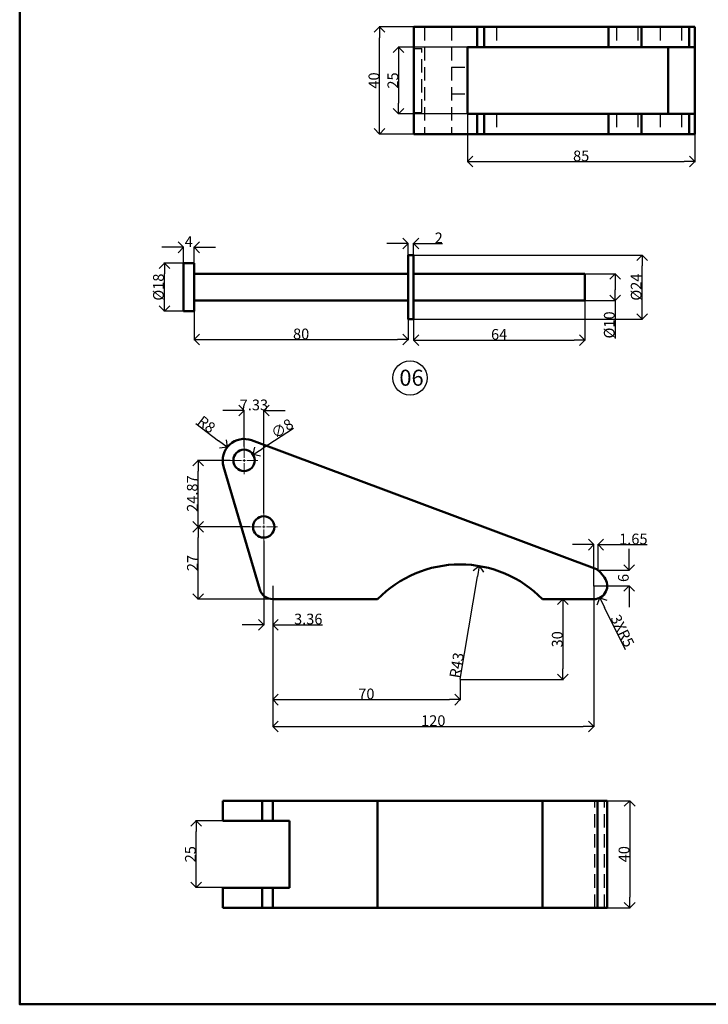
# Model space of a CAD drawing. Units: millimetres. Extents: x 45 to 546, y 51 to 638.
# Tile 1 of 4: x 45 to 303, y 51 to 419. Entities that reach past the tile are written whole.
import ezdxf

# ---------------------------------------------------------------- set-up
doc = ezdxf.new("R2010")
doc.units = ezdxf.units.MM
doc.header["$MEASUREMENT"] = 0
doc.linetypes.add('CENTER2', pattern=[1.125, 0.75, -0.125, 0.125, -0.125])
doc.linetypes.add('HIDDEN', pattern=[0.375, 0.25, -0.125])
for name, color, linetype, lineweight in [('M-CNTR', 1, 'CENTER2', 18), ('M-DIMS', 2, 'Continuous', 25), ('M-HIDN', 8, 'HIDDEN', 25), ('M-OUTL', 7, 'Continuous', 50), ('M-TEXT', 7, 'Continuous', 25), ('M-TTLB', 7, 'Continuous', 50)]:
    doc.layers.add(name, color=color, linetype=linetype, lineweight=lineweight)
doc.styles.get("Standard").update_dxf_attribs({"font": 'arial.ttf'})
doc.dimstyles.get("Standard").update_dxf_attribs({"dimtxt": 4, "dimasz": 4, "dimexe": 0.18, "dimexo": 0.0625, "dimgap": 0.09, "dimtad": 1, "dimdec": 0, "dimzin": 0, "dimdsep": 46, "dimtxsty": 'Standard', "dimblk": 'OPEN90', "dimcen": 0.09, "dimclre": 251, "dimadec": 0, "dimazin": 0, "dimtfac": 1, "dimtdec": 0, "dimtofl": 0, "dimtmove": 0, "dimatfit": 3, "dimfxl": 1, "dimtolj": 1, "dimtzin": 0, "dimarcsym": 0})

# ---------------------------------------------------------------- blocks, each defined once
blk = doc.blocks.new('_Open90')
at = {"color": 0, "linetype": 'ByBlock', "lineweight": -2}
for p, q in [((0, 0), (-1, 0)), ((-0.5, 0.5), (0, 0)), ((0, 0), (-0.5, -0.5))]:
    blk.add_line(p, q, dxfattribs=at)
blk = doc.blocks.new('*D28')
at = {"layer": 'Defpoints', "color": 0, "transparency": 16777216}
for p in [(179.84, 416.24), (192.68, 416.24), (192.68, 376.24)]:
    blk.add_point(p, dxfattribs=at)
at = {"layer": 'M-DIMS', "color": 0, "lineweight": -2, "transparency": 16777216}
for p, q in [((192.61, 416.24), (179.66, 416.24)), ((179.84, 380.24), (179.84, 412.24)), ((192.61, 376.24), (179.66, 376.24))]:
    blk.add_line(p, q, dxfattribs=at)
at = {"layer": 'M-DIMS', "color": 0, "lineweight": -2, "transparency": 16777216, "xscale": 4, "yscale": 4, "zscale": 4}
for p, rotation in [((179.84, 416.24), 90), ((179.84, 376.24), 270)]:
    blk.add_blockref('_Open90', p, dxfattribs=dict(at, rotation=rotation))
at = {"layer": 'M-DIMS', "color": 0, "transparency": 16777216, "insert": (177.71, 396.24), "char_height": 4, "attachment_point": 5, "rotation": 90}
blk.add_mtext('\\A1;40', dxfattribs=at)
blk = doc.blocks.new('*D29')
at = {"layer": 'Defpoints', "color": 0, "transparency": 16777216}
for p in [(212.68, 408.74), (186.92, 383.74), (212.68, 383.74)]:
    blk.add_point(p, dxfattribs=at)
at = {"layer": 'M-DIMS', "color": 0, "lineweight": -2, "transparency": 16777216}
for p, q in [((212.61, 408.74), (186.74, 408.74)), ((186.92, 404.74), (186.92, 387.74)), ((212.61, 383.74), (186.74, 383.74))]:
    blk.add_line(p, q, dxfattribs=at)
at = {"layer": 'M-DIMS', "color": 0, "lineweight": -2, "transparency": 16777216, "xscale": 4, "yscale": 4, "zscale": 4}
for p, rotation in [((186.92, 408.74), 90), ((186.92, 383.74), 270)]:
    blk.add_blockref('_Open90', p, dxfattribs=dict(at, rotation=rotation))
at = {"layer": 'M-DIMS', "color": 0, "transparency": 16777216, "insert": (184.79, 396.24), "char_height": 4, "attachment_point": 5, "rotation": 90}
blk.add_mtext('\\A1;25', dxfattribs=at)
blk = doc.blocks.new('*D30')
at = {"layer": 'Defpoints', "color": 0, "transparency": 16777216}
for p in [(212.68, 383.74), (297.68, 383.74), (297.68, 365.93)]:
    blk.add_point(p, dxfattribs=at)
at = {"layer": 'M-DIMS', "color": 0, "lineweight": -2, "transparency": 16777216}
for p, q in [((212.68, 383.68), (212.68, 365.75)), ((297.68, 383.68), (297.68, 365.75)), ((216.68, 365.93), (293.68, 365.93))]:
    blk.add_line(p, q, dxfattribs=at)
at = {"layer": 'M-DIMS', "color": 0, "lineweight": -2, "transparency": 16777216, "xscale": 4, "yscale": 4, "zscale": 4, "rotation": 180}
blk.add_blockref('_Open90', (212.68, 365.93), dxfattribs=at)
at = {"layer": 'M-DIMS', "color": 0, "lineweight": -2, "transparency": 16777216, "xscale": 4, "yscale": 4, "zscale": 4}
blk.add_blockref('_Open90', (297.68, 365.93), dxfattribs=at)
at = {"layer": 'M-DIMS', "color": 0, "transparency": 16777216, "insert": (255.18, 368.06), "char_height": 4, "attachment_point": 5}
blk.add_mtext('\\A1;85', dxfattribs=at)
blk = doc.blocks.new('*D77')
at = {"layer": 'Defpoints', "color": 0, "transparency": 16777216}
for p in [(99.44, 328.03), (106.53, 328.03), (106.53, 310.03)]:
    blk.add_point(p, dxfattribs=at)
at = {"layer": 'M-DIMS', "color": 0, "lineweight": -2, "transparency": 16777216}
for p, q in [((106.46, 328.03), (99.26, 328.03)), ((99.44, 314.03), (99.44, 324.03)), ((106.46, 310.03), (99.26, 310.03))]:
    blk.add_line(p, q, dxfattribs=at)
at = {"layer": 'M-DIMS', "color": 0, "lineweight": -2, "transparency": 16777216, "xscale": 4, "yscale": 4, "zscale": 4}
for p, rotation in [((99.44, 328.03), 90), ((99.44, 310.03), 270)]:
    blk.add_blockref('_Open90', p, dxfattribs=dict(at, rotation=rotation))
at = {"layer": 'M-DIMS', "color": 0, "transparency": 16777216, "insert": (97.2, 319.03), "char_height": 4, "attachment_point": 5, "rotation": 90}
blk.add_mtext('\\A1;%%C18', dxfattribs=at)
blk = doc.blocks.new('*D78')
at = {"layer": 'Defpoints', "color": 0, "transparency": 16777216}
for p in [(110.53, 333.9), (106.53, 328.03), (110.53, 328.03)]:
    blk.add_point(p, dxfattribs=at)
at = {"layer": 'M-DIMS', "color": 0, "lineweight": -2, "transparency": 16777216}
for p, q in [((102.53, 333.9), (98.53, 333.9)), ((106.53, 328.09), (106.53, 334.08)), ((110.53, 328.09), (110.53, 334.08)), ((114.53, 333.9), (118.53, 333.9))]:
    blk.add_line(p, q, dxfattribs=at)
at = {"layer": 'M-DIMS', "color": 0, "lineweight": -2, "transparency": 16777216, "xscale": 4, "yscale": 4, "zscale": 4}
blk.add_blockref('_Open90', (106.53, 333.9), dxfattribs=at)
at = {"layer": 'M-DIMS', "color": 0, "lineweight": -2, "transparency": 16777216, "xscale": 4, "yscale": 4, "zscale": 4, "rotation": 180}
blk.add_blockref('_Open90', (110.53, 333.9), dxfattribs=at)
at = {"layer": 'M-DIMS', "color": 0, "transparency": 16777216, "insert": (108.53, 335.99), "char_height": 4, "attachment_point": 5}
blk.add_mtext('\\A1;4', dxfattribs=at)
blk = doc.blocks.new('*D79')
at = {"layer": 'Defpoints', "color": 0, "transparency": 16777216}
for p in [(192.53, 335.33), (190.53, 331.03), (192.53, 331.03)]:
    blk.add_point(p, dxfattribs=at)
at = {"layer": 'M-DIMS', "color": 0, "lineweight": -2, "transparency": 16777216}
for p, q in [((186.53, 335.33), (182.53, 335.33)), ((190.53, 331.09), (190.53, 335.51)), ((192.53, 331.09), (192.53, 335.51)), ((196.53, 335.33), (203.36, 335.33))]:
    blk.add_line(p, q, dxfattribs=at)
at = {"layer": 'M-DIMS', "color": 0, "lineweight": -2, "transparency": 16777216, "xscale": 4, "yscale": 4, "zscale": 4}
blk.add_blockref('_Open90', (190.53, 335.33), dxfattribs=at)
at = {"layer": 'M-DIMS', "color": 0, "lineweight": -2, "transparency": 16777216, "xscale": 4, "yscale": 4, "zscale": 4, "rotation": 180}
blk.add_blockref('_Open90', (192.53, 335.33), dxfattribs=at)
at = {"layer": 'M-DIMS', "color": 0, "transparency": 16777216, "insert": (201.94, 337.43), "char_height": 4, "attachment_point": 5}
blk.add_mtext('\\A1;2', dxfattribs=at)
blk = doc.blocks.new('*D80')
at = {"layer": 'Defpoints', "color": 0, "transparency": 16777216}
for p in [(110.53, 310.03), (190.53, 307.03), (190.53, 299.42)]:
    blk.add_point(p, dxfattribs=at)
at = {"layer": 'M-DIMS', "color": 0, "lineweight": -2, "transparency": 16777216}
for p, q in [((110.53, 309.96), (110.53, 299.24)), ((190.53, 306.96), (190.53, 299.24)), ((114.53, 299.42), (186.53, 299.42))]:
    blk.add_line(p, q, dxfattribs=at)
at = {"layer": 'M-DIMS', "color": 0, "lineweight": -2, "transparency": 16777216, "xscale": 4, "yscale": 4, "zscale": 4, "rotation": 180}
blk.add_blockref('_Open90', (110.53, 299.42), dxfattribs=at)
at = {"layer": 'M-DIMS', "color": 0, "lineweight": -2, "transparency": 16777216, "xscale": 4, "yscale": 4, "zscale": 4}
blk.add_blockref('_Open90', (190.53, 299.42), dxfattribs=at)
at = {"layer": 'M-DIMS', "color": 0, "transparency": 16777216, "insert": (150.53, 301.55), "char_height": 4, "attachment_point": 5}
blk.add_mtext('\\A1;80', dxfattribs=at)
blk = doc.blocks.new('*D81')
at = {"layer": 'Defpoints', "color": 0, "transparency": 16777216}
for p in [(256.53, 314.03), (192.53, 307.03), (256.53, 299.24)]:
    blk.add_point(p, dxfattribs=at)
at = {"layer": 'M-DIMS', "color": 0, "lineweight": -2, "transparency": 16777216}
for p, q in [((256.53, 313.96), (256.53, 299.06)), ((192.53, 306.96), (192.53, 299.06)), ((196.53, 299.24), (252.53, 299.24))]:
    blk.add_line(p, q, dxfattribs=at)
at = {"layer": 'M-DIMS', "color": 0, "lineweight": -2, "transparency": 16777216, "xscale": 4, "yscale": 4, "zscale": 4, "rotation": 180}
blk.add_blockref('_Open90', (192.53, 299.24), dxfattribs=at)
at = {"layer": 'M-DIMS', "color": 0, "lineweight": -2, "transparency": 16777216, "xscale": 4, "yscale": 4, "zscale": 4}
blk.add_blockref('_Open90', (256.53, 299.24), dxfattribs=at)
at = {"layer": 'M-DIMS', "color": 0, "transparency": 16777216, "insert": (224.53, 301.37), "char_height": 4, "attachment_point": 5}
blk.add_mtext('\\A1;64', dxfattribs=at)
blk = doc.blocks.new('*D82')
at = {"layer": 'Defpoints', "color": 0, "transparency": 16777216}
for p in [(256.53, 324.03), (256.53, 314.03), (267.91, 314.03)]:
    blk.add_point(p, dxfattribs=at)
at = {"layer": 'M-DIMS', "color": 0, "lineweight": -2, "transparency": 16777216}
for p, q in [((256.59, 324.03), (268.09, 324.03)), ((267.91, 320.03), (267.91, 318.03)), ((256.59, 314.03), (268.09, 314.03)), ((267.91, 314.03), (267.91, 299.78))]:
    blk.add_line(p, q, dxfattribs=at)
at = {"layer": 'M-DIMS', "color": 0, "lineweight": -2, "transparency": 16777216, "xscale": 4, "yscale": 4, "zscale": 4}
for p, rotation in [((267.91, 324.03), 90), ((267.91, 314.03), 270)]:
    blk.add_blockref('_Open90', p, dxfattribs=dict(at, rotation=rotation))
at = {"layer": 'M-DIMS', "color": 0, "transparency": 16777216, "insert": (265.67, 304.9), "char_height": 4, "attachment_point": 5, "rotation": 90}
blk.add_mtext('\\A1;%%C10', dxfattribs=at)
blk = doc.blocks.new('*D83')
at = {"layer": 'Defpoints', "color": 0, "transparency": 16777216}
for p in [(192.53, 331.03), (277.97, 331.03), (192.53, 307.03)]:
    blk.add_point(p, dxfattribs=at)
at = {"layer": 'M-DIMS', "color": 0, "lineweight": -2, "transparency": 16777216}
for p, q in [((192.59, 331.03), (278.15, 331.03)), ((277.97, 311.03), (277.97, 327.03)), ((192.59, 307.03), (278.15, 307.03))]:
    blk.add_line(p, q, dxfattribs=at)
at = {"layer": 'M-DIMS', "color": 0, "lineweight": -2, "transparency": 16777216, "xscale": 4, "yscale": 4, "zscale": 4}
for p, rotation in [((277.97, 331.03), 90), ((277.97, 307.03), 270)]:
    blk.add_blockref('_Open90', p, dxfattribs=dict(at, rotation=rotation))
at = {"layer": 'M-DIMS', "color": 0, "transparency": 16777216, "insert": (275.73, 319.03), "char_height": 4, "attachment_point": 5, "rotation": 90}
blk.add_mtext('\\A1;%%C24', dxfattribs=at)
blk = doc.blocks.new('*U84')
at = {"layer": 'M-CNTR', "color": 0, "transparency": 16777216}
for p, q in [((0, 1), (0, 5.12)), ((-5.12, 0), (-1, 0)), ((1, 0), (5.12, 0)), ((0, -5.12), (0, -1))]:
    blk.add_line(p, q, dxfattribs=at)
at = {"layer": 'M-CNTR', "color": 0, "linetype": 'Continuous', "transparency": 16777216}
for p, q in [((-0.5, 0), (0.5, 0)), ((0, -0.5), (0, 0.5))]:
    blk.add_line(p, q, dxfattribs=at)
blk = doc.blocks.new('*U85')
at = {"layer": 'M-CNTR', "color": 0, "transparency": 16777216}
for p, q in [((0, 1), (0, 5.12)), ((-5.12, 0), (-1, 0)), ((1, 0), (5.12, 0)), ((0, -5.12), (0, -1))]:
    blk.add_line(p, q, dxfattribs=at)
at = {"layer": 'M-CNTR', "color": 0, "linetype": 'Continuous', "transparency": 16777216}
for p, q in [((-0.5, 0), (0.5, 0)), ((0, -0.5), (0, 0.5))]:
    blk.add_line(p, q, dxfattribs=at)
blk = doc.blocks.new('*D86')
at = {"layer": 'Defpoints', "color": 0, "transparency": 16777216}
for p in [(112, 229.43), (131.43, 229.43), (139.91, 202.43)]:
    blk.add_point(p, dxfattribs=at)
at = {"layer": 'M-DIMS', "color": 0, "lineweight": -2, "transparency": 16777216}
for p, q in [((131.37, 229.43), (111.82, 229.43)), ((112, 206.43), (112, 225.43)), ((139.85, 202.43), (111.82, 202.43))]:
    blk.add_line(p, q, dxfattribs=at)
at = {"layer": 'M-DIMS', "color": 0, "lineweight": -2, "transparency": 16777216, "xscale": 4, "yscale": 4, "zscale": 4}
for p, rotation in [((112, 229.43), 90), ((112, 202.43), 270)]:
    blk.add_blockref('_Open90', p, dxfattribs=dict(at, rotation=rotation))
at = {"layer": 'M-DIMS', "color": 0, "transparency": 16777216, "insert": (109.9, 215.93), "char_height": 4, "attachment_point": 5, "rotation": 90}
blk.add_mtext('\\A1;27', dxfattribs=at)
blk = doc.blocks.new('*D87')
at = {"layer": 'Defpoints', "color": 0, "transparency": 16777216}
for p in [(112, 254.3), (124.1, 254.3), (131.43, 229.43)]:
    blk.add_point(p, dxfattribs=at)
at = {"layer": 'M-DIMS', "color": 0, "lineweight": -2, "transparency": 16777216}
for p, q in [((124.04, 254.3), (111.82, 254.3)), ((112, 233.43), (112, 250.3)), ((131.37, 229.43), (111.82, 229.43))]:
    blk.add_line(p, q, dxfattribs=at)
at = {"layer": 'M-DIMS', "color": 0, "lineweight": -2, "transparency": 16777216, "xscale": 4, "yscale": 4, "zscale": 4}
for p, rotation in [((112, 254.3), 90), ((112, 229.43), 270)]:
    blk.add_blockref('_Open90', p, dxfattribs=dict(at, rotation=rotation))
at = {"layer": 'M-DIMS', "color": 0, "transparency": 16777216, "insert": (109.86, 241.87), "char_height": 4, "attachment_point": 5, "rotation": 90}
blk.add_mtext('\\A1;24.87', dxfattribs=at)
blk = doc.blocks.new('*D88')
at = {"layer": 'Defpoints', "color": 0, "transparency": 16777216}
for p in [(129.22, 272.89), (129.22, 259.42), (136.55, 234.55)]:
    blk.add_point(p, dxfattribs=at)
at = {"layer": 'M-DIMS', "color": 0, "lineweight": -2, "transparency": 16777216}
for p, q in [((125.22, 272.89), (121.22, 272.89)), ((129.22, 259.49), (129.22, 273.07)), ((136.55, 234.62), (136.55, 273.07)), ((140.55, 272.89), (144.55, 272.89))]:
    blk.add_line(p, q, dxfattribs=at)
at = {"layer": 'M-DIMS', "color": 0, "lineweight": -2, "transparency": 16777216, "xscale": 4, "yscale": 4, "zscale": 4}
blk.add_blockref('_Open90', (129.22, 272.89), dxfattribs=at)
at = {"layer": 'M-DIMS', "color": 0, "lineweight": -2, "transparency": 16777216, "xscale": 4, "yscale": 4, "zscale": 4, "rotation": 180}
blk.add_blockref('_Open90', (136.55, 272.89), dxfattribs=at)
at = {"layer": 'M-DIMS', "color": 0, "transparency": 16777216, "insert": (132.88, 275.02), "char_height": 4, "attachment_point": 5}
blk.add_mtext('\\A1;7.33', dxfattribs=at)
blk = doc.blocks.new('*D89')
at = {"layer": 'Defpoints', "color": 0, "transparency": 16777216}
for p in [(122.86, 259.17), (129.22, 254.3)]:
    blk.add_point(p, dxfattribs=at)
at = {"layer": 'M-DIMS', "color": 0, "lineweight": -2, "transparency": 16777216}
for p, q in [((111.24, 268.06), (119.69, 261.6)), ((129.13, 254.3), (129.31, 254.3)), ((129.22, 254.21), (129.22, 254.39))]:
    blk.add_line(p, q, dxfattribs=at)
at = {"layer": 'M-DIMS', "color": 0, "lineweight": -2, "transparency": 16777216, "xscale": 4, "yscale": 4, "zscale": 4, "rotation": 322.5817597606711}
blk.add_blockref('_Open90', (122.86, 259.17), dxfattribs=at)
at = {"layer": 'M-DIMS', "color": 0, "transparency": 16777216, "insert": (115.17, 267.74), "char_height": 4, "attachment_point": 5, "rotation": 322.5818}
blk.add_mtext('\\A1;R8', dxfattribs=at)
blk = doc.blocks.new('*D90')
at = {"layer": 'Defpoints', "color": 0, "transparency": 16777216}
for p in [(132.58, 256.48), (125.86, 252.13)]:
    blk.add_point(p, dxfattribs=at)
at = {"layer": 'M-DIMS', "color": 0, "lineweight": -2, "transparency": 16777216}
for p, q in [((147.67, 266.24), (135.93, 258.65)), ((129.13, 254.3), (129.31, 254.3)), ((129.22, 254.21), (129.22, 254.39))]:
    blk.add_line(p, q, dxfattribs=at)
at = {"layer": 'M-DIMS', "color": 0, "lineweight": -2, "transparency": 16777216, "xscale": 4, "yscale": 4, "zscale": 4, "rotation": 212.9103670149516}
blk.add_blockref('_Open90', (132.58, 256.48), dxfattribs=at)
at = {"layer": 'M-DIMS', "color": 0, "transparency": 16777216, "insert": (143.44, 266.18), "char_height": 4, "attachment_point": 5, "rotation": 32.9104}
blk.add_mtext('\\A1;∅8', dxfattribs=at)
blk = doc.blocks.new('*D91')
at = {"layer": 'Defpoints', "color": 0, "transparency": 16777216}
for p in [(136.55, 224.31), (139.91, 207.43), (139.91, 192.87)]:
    blk.add_point(p, dxfattribs=at)
at = {"layer": 'M-DIMS', "color": 0, "lineweight": -2, "transparency": 16777216}
for p, q in [((136.55, 224.25), (136.55, 192.69)), ((139.91, 207.37), (139.91, 192.69)), ((132.55, 192.87), (128.55, 192.87)), ((143.91, 192.87), (158.47, 192.87))]:
    blk.add_line(p, q, dxfattribs=at)
at = {"layer": 'M-DIMS', "color": 0, "lineweight": -2, "transparency": 16777216, "xscale": 4, "yscale": 4, "zscale": 4}
blk.add_blockref('_Open90', (136.55, 192.87), dxfattribs=at)
at = {"layer": 'M-DIMS', "color": 0, "lineweight": -2, "transparency": 16777216, "xscale": 4, "yscale": 4, "zscale": 4, "rotation": 180}
blk.add_blockref('_Open90', (139.91, 192.87), dxfattribs=at)
at = {"layer": 'M-DIMS', "color": 0, "transparency": 16777216, "insert": (153.19, 195.01), "char_height": 4, "attachment_point": 5}
blk.add_mtext('\\A1;3.36', dxfattribs=at)
blk = doc.blocks.new('*D92')
at = {"layer": 'Defpoints', "color": 0, "transparency": 16777216}
for p in [(139.91, 207.43), (209.91, 172.43), (209.91, 164.89)]:
    blk.add_point(p, dxfattribs=at)
at = {"layer": 'M-DIMS', "color": 0, "lineweight": -2, "transparency": 16777216}
for p, q in [((139.91, 207.37), (139.91, 164.71)), ((209.91, 172.37), (209.91, 164.71)), ((143.91, 164.89), (205.91, 164.89))]:
    blk.add_line(p, q, dxfattribs=at)
at = {"layer": 'M-DIMS', "color": 0, "lineweight": -2, "transparency": 16777216, "xscale": 4, "yscale": 4, "zscale": 4, "rotation": 180}
blk.add_blockref('_Open90', (139.91, 164.89), dxfattribs=at)
at = {"layer": 'M-DIMS', "color": 0, "lineweight": -2, "transparency": 16777216, "xscale": 4, "yscale": 4, "zscale": 4}
blk.add_blockref('_Open90', (209.91, 164.89), dxfattribs=at)
at = {"layer": 'M-DIMS', "color": 0, "transparency": 16777216, "insert": (174.91, 167.03), "char_height": 4, "attachment_point": 5}
blk.add_mtext('\\A1;70', dxfattribs=at)
blk = doc.blocks.new('*D93')
at = {"layer": 'Defpoints', "color": 0, "transparency": 16777216}
for p in [(245.97, 202.43), (209.91, 172.43), (248.37, 172.43)]:
    blk.add_point(p, dxfattribs=at)
at = {"layer": 'M-DIMS', "color": 0, "lineweight": -2, "transparency": 16777216}
for p, q in [((246.04, 202.43), (248.55, 202.43)), ((248.37, 198.43), (248.37, 176.43)), ((209.97, 172.43), (248.55, 172.43))]:
    blk.add_line(p, q, dxfattribs=at)
at = {"layer": 'M-DIMS', "color": 0, "lineweight": -2, "transparency": 16777216, "xscale": 4, "yscale": 4, "zscale": 4}
for p, rotation in [((248.37, 202.43), 90), ((248.37, 172.43), 270)]:
    blk.add_blockref('_Open90', p, dxfattribs=dict(at, rotation=rotation))
at = {"layer": 'M-DIMS', "color": 0, "transparency": 16777216, "insert": (246.23, 187.43), "char_height": 4, "attachment_point": 5, "rotation": 90}
blk.add_mtext('\\A1;30', dxfattribs=at)
blk = doc.blocks.new('*D94')
at = {"layer": 'Defpoints', "color": 0, "transparency": 16777216}
for p in [(139.91, 207.43), (259.91, 207.43), (259.91, 154.91)]:
    blk.add_point(p, dxfattribs=at)
at = {"layer": 'M-DIMS', "color": 0, "lineweight": -2, "transparency": 16777216}
for p, q in [((139.91, 207.37), (139.91, 154.73)), ((259.91, 207.37), (259.91, 154.73)), ((143.91, 154.91), (255.91, 154.91))]:
    blk.add_line(p, q, dxfattribs=at)
at = {"layer": 'M-DIMS', "color": 0, "lineweight": -2, "transparency": 16777216, "xscale": 4, "yscale": 4, "zscale": 4, "rotation": 180}
blk.add_blockref('_Open90', (139.91, 154.91), dxfattribs=at)
at = {"layer": 'M-DIMS', "color": 0, "lineweight": -2, "transparency": 16777216, "xscale": 4, "yscale": 4, "zscale": 4}
blk.add_blockref('_Open90', (259.91, 154.91), dxfattribs=at)
at = {"layer": 'M-DIMS', "color": 0, "transparency": 16777216, "insert": (199.91, 157.04), "char_height": 4, "attachment_point": 5}
blk.add_mtext('\\A1;120', dxfattribs=at)
blk = doc.blocks.new('*D95')
at = {"layer": 'Defpoints', "color": 0, "transparency": 16777216}
for p in [(217.1, 214.83), (209.91, 172.43)]:
    blk.add_point(p, dxfattribs=at)
at = {"layer": 'M-DIMS', "color": 0, "lineweight": -2, "transparency": 16777216}
blk.add_line((209.93, 172.57), (216.43, 210.89), dxfattribs=at)
at = {"layer": 'M-DIMS', "color": 0, "lineweight": -2, "transparency": 16777216, "xscale": 4, "yscale": 4, "zscale": 4, "rotation": 80.37551850452407}
blk.add_blockref('_Open90', (217.1, 214.83), dxfattribs=at)
at = {"layer": 'M-DIMS', "color": 0, "transparency": 16777216, "insert": (208.64, 177.73), "char_height": 4, "attachment_point": 5, "rotation": 80.3755}
blk.add_mtext('\\A1;R43', dxfattribs=at)
blk = doc.blocks.new('*D96')
at = {"layer": 'Defpoints', "color": 0, "transparency": 16777216}
for p in [(261.45, 213.29), (273.08, 213.29), (259.91, 207.43)]:
    blk.add_point(p, dxfattribs=at)
at = {"layer": 'M-DIMS', "color": 0, "lineweight": -2, "transparency": 16777216}
for p, q in [((273.08, 217.29), (273.08, 221.29)), ((261.51, 213.29), (273.26, 213.29)), ((259.97, 207.43), (273.26, 207.43)), ((273.08, 203.43), (273.08, 199.43))]:
    blk.add_line(p, q, dxfattribs=at)
at = {"layer": 'M-DIMS', "color": 0, "lineweight": -2, "transparency": 16777216, "xscale": 4, "yscale": 4, "zscale": 4}
for p, rotation in [((273.08, 213.29), 270), ((273.08, 207.43), 90)]:
    blk.add_blockref('_Open90', p, dxfattribs=dict(at, rotation=rotation))
at = {"layer": 'M-DIMS', "color": 0, "transparency": 16777216, "insert": (270.95, 210.36), "char_height": 4, "attachment_point": 5, "rotation": 90}
blk.add_mtext('\\A1;6', dxfattribs=at)
blk = doc.blocks.new('*D97')
at = {"layer": 'Defpoints', "color": 0, "transparency": 16777216}
for p in [(261.56, 222.8), (261.56, 213.2), (259.91, 207.43)]:
    blk.add_point(p, dxfattribs=at)
at = {"layer": 'M-DIMS', "color": 0, "lineweight": -2, "transparency": 16777216}
for p, q in [((255.91, 222.8), (251.91, 222.8)), ((259.91, 207.5), (259.91, 222.98)), ((261.56, 213.27), (261.56, 222.98)), ((265.56, 222.8), (279.78, 222.8))]:
    blk.add_line(p, q, dxfattribs=at)
at = {"layer": 'M-DIMS', "color": 0, "lineweight": -2, "transparency": 16777216, "xscale": 4, "yscale": 4, "zscale": 4}
blk.add_blockref('_Open90', (259.91, 222.8), dxfattribs=at)
at = {"layer": 'M-DIMS', "color": 0, "lineweight": -2, "transparency": 16777216, "xscale": 4, "yscale": 4, "zscale": 4, "rotation": 180}
blk.add_blockref('_Open90', (261.56, 222.8), dxfattribs=at)
at = {"layer": 'M-DIMS', "color": 0, "transparency": 16777216, "insert": (274.67, 224.93), "char_height": 4, "attachment_point": 5}
blk.add_mtext('\\A1;1.65', dxfattribs=at)
blk = doc.blocks.new('*D98')
at = {"layer": 'Defpoints', "color": 0, "transparency": 16777216}
for p in [(259.91, 207.43), (262.12, 202.95)]:
    blk.add_point(p, dxfattribs=at)
at = {"layer": 'M-DIMS', "color": 0, "lineweight": -2, "transparency": 16777216}
for p, q in [((259.82, 207.43), (260, 207.43)), ((259.91, 207.34), (259.91, 207.52)), ((271.74, 183.5), (263.9, 199.37))]:
    blk.add_line(p, q, dxfattribs=at)
at = {"layer": 'M-DIMS', "color": 0, "lineweight": -2, "transparency": 16777216, "xscale": 4, "yscale": 4, "zscale": 4, "rotation": 116.3040513047438}
blk.add_blockref('_Open90', (262.12, 202.95), dxfattribs=at)
at = {"layer": 'M-DIMS', "color": 0, "transparency": 16777216, "insert": (270.62, 190.59), "char_height": 4, "attachment_point": 5, "rotation": 296.3041}
blk.add_mtext('\\A1;3XR5', dxfattribs=at)
blk = doc.blocks.new('*D99')
at = {"layer": 'Defpoints', "color": 0, "transparency": 16777216}
for p in [(111.27, 119.64), (121.22, 119.64), (121.22, 94.64)]:
    blk.add_point(p, dxfattribs=at)
at = {"layer": 'M-DIMS', "color": 0, "lineweight": -2, "transparency": 16777216}
for p, q in [((121.16, 119.64), (111.09, 119.64)), ((111.27, 98.64), (111.27, 115.64)), ((121.16, 94.64), (111.09, 94.64))]:
    blk.add_line(p, q, dxfattribs=at)
at = {"layer": 'M-DIMS', "color": 0, "lineweight": -2, "transparency": 16777216, "xscale": 4, "yscale": 4, "zscale": 4}
for p, rotation in [((111.27, 119.64), 90), ((111.27, 94.64), 270)]:
    blk.add_blockref('_Open90', p, dxfattribs=dict(at, rotation=rotation))
at = {"layer": 'M-DIMS', "color": 0, "transparency": 16777216, "insert": (109.13, 107.14), "char_height": 4, "attachment_point": 5, "rotation": 90}
blk.add_mtext('\\A1;25', dxfattribs=at)
blk = doc.blocks.new('*D100')
at = {"layer": 'Defpoints', "color": 0, "transparency": 16777216}
for p in [(264.91, 127.14), (264.91, 87.14), (273.3, 87.14)]:
    blk.add_point(p, dxfattribs=at)
at = {"layer": 'M-DIMS', "color": 0, "lineweight": -2, "transparency": 16777216}
for p, q in [((264.97, 127.14), (273.48, 127.14)), ((273.3, 123.14), (273.3, 91.14)), ((264.97, 87.14), (273.48, 87.14))]:
    blk.add_line(p, q, dxfattribs=at)
at = {"layer": 'M-DIMS', "color": 0, "lineweight": -2, "transparency": 16777216, "xscale": 4, "yscale": 4, "zscale": 4}
for p, rotation in [((273.3, 127.14), 90), ((273.3, 87.14), 270)]:
    blk.add_blockref('_Open90', p, dxfattribs=dict(at, rotation=rotation))
at = {"layer": 'M-DIMS', "color": 0, "transparency": 16777216, "insert": (271.17, 107.14), "char_height": 4, "attachment_point": 5, "rotation": 90}
blk.add_mtext('\\A1;40', dxfattribs=at)

msp = doc.modelspace()

# ---------------------------------------------------------------- linework, layer by layer
at = {"layer": 'M-HIDN', "ltscale": 20}
for p, q in [((196.676, 416.24), (196.676, 376.24)), ((206.676, 416.24), (206.676, 376.24)), ((223.526, 416.24), (223.526, 408.74)), ((268.326, 416.24), (268.326, 408.74)), ((276.326, 416.24), (276.326, 408.74)), ((284.676, 416.24), (284.676, 408.74)), ((292.676, 416.24), (292.676, 408.74)), ((192.676, 408.24), (195.676, 408.24)), ((195.676, 384.24), (195.676, 408.24)), ((206.676, 401.24), (212.676, 401.24)), ((206.676, 391.24), (212.676, 391.24)), ((192.676, 384.24), (195.676, 384.24)), ((223.526, 383.74), (223.526, 376.24)), ((268.326, 383.74), (268.326, 376.24)), ((276.326, 383.74), (276.326, 376.24)), ((284.676, 383.74), (284.676, 376.24)), ((292.676, 383.74), (292.676, 376.24)), ((260.284, 87.135), (260.284, 127.135)), ((263.844, 87.135), (263.844, 127.135))]:
    msp.add_line(p, q, dxfattribs=at)
at = {"layer": 'M-OUTL'}
for p, q in [((192.676, 416.24), (192.676, 376.24)), ((297.676, 416.24), (192.676, 416.24)), ((216.283, 416.24), (216.283, 408.74)), ((218.868, 416.24), (218.868, 408.74)), ((265.422, 408.74), (265.422, 416.24)), ((277.676, 408.74), (277.676, 416.24)), ((295.58, 416.24), (295.58, 408.74)), ((297.676, 416.24), (297.676, 376.24)), ((212.676, 408.74), (212.676, 383.74)), ((212.676, 408.74), (297.676, 408.74)), ((287.676, 408.74), (287.676, 383.74)), ((212.676, 383.74), (297.676, 383.74)), ((216.283, 383.74), (216.283, 376.24)), ((218.868, 383.74), (218.868, 376.24)), ((265.422, 383.74), (265.422, 376.24)), ((277.676, 383.74), (277.676, 376.24)), ((295.58, 383.74), (295.58, 376.24)), ((297.676, 376.24), (192.676, 376.24)), ((106.527, 310.027), (106.527, 328.027)), ((106.527, 328.027), (110.527, 328.027)), ((110.527, 328.027), (110.527, 310.027)), ((110.527, 324.027), (190.527, 324.027)), ((192.527, 324.027), (256.527, 324.027)), ((256.527, 314.027), (256.527, 324.027)), ((110.527, 314.027), (190.527, 314.027)), ((192.527, 314.027), (256.527, 314.027)), ((110.527, 310.027), (106.527, 310.027)), ((132.016, 261.8), (260.284, 213.932)), ((121.545, 252.042), (135.096, 206.079)), ((262.403, 212.358), (263.844, 210.519)), ((139.909, 202.435), (179.103, 202.435)), ((240.715, 202.435), (259.909, 202.435)), ((121.219, 127.135), (121.219, 119.635)), ((121.219, 127.135), (264.909, 127.135)), ((135.935, 127.135), (135.935, 119.635)), ((139.909, 127.135), (139.909, 119.635)), ((179.103, 127.135), (179.103, 87.135)), ((240.715, 127.135), (240.715, 87.135)), ((261.222, 127.135), (261.222, 87.135)), ((264.909, 127.135), (264.909, 87.135)), ((146.219, 119.635), (121.219, 119.635)), ((146.219, 119.635), (146.219, 94.635)), ((146.219, 94.635), (121.219, 94.635)), ((121.219, 94.635), (121.219, 87.135)), ((135.935, 94.635), (135.935, 87.135)), ((139.909, 94.635), (139.909, 87.135)), ((121.219, 87.135), (264.909, 87.135))]:
    msp.add_line(p, q, dxfattribs=at)
msp.add_lwpolyline([(190.527, 331.027), (192.527, 331.027), (192.527, 307.027), (190.527, 307.027)], close=True, dxfattribs=at)
for centre in [(129.219, 254.305), (136.549, 229.435)]:
    msp.add_circle(centre, 4, dxfattribs=at)
for centre, radius, start, end in [((129.219, 254.305), 8, 69.53501, 196.42637), ((209.909, 172.435), 43, 44.24072, 135.75928), ((258.468, 209.273), 5, 38.08982, 68.7041), ((259.909, 207.435), 5, 270, 38.08982), ((139.909, 207.435), 5, 195.73592, 270)]:
    msp.add_arc(centre, radius, start, end, dxfattribs=at)
at = {"layer": 'M-TEXT'}
msp.add_circle((191.214, 285.08), 6.408, dxfattribs=at)
at = {"layer": 'M-TTLB'}
msp.add_lwpolyline([(45.357, 637.893), (546.237, 637.893), (546.237, 51.054), (45.357, 51.054)], close=True, dxfattribs=at)

# ---------------------------------------------------------------- block references
at = {"layer": 'M-CNTR'}
for name, p in [('*U85', (129.219, 254.305)), ('*U84', (136.549, 229.435))]:
    msp.add_blockref(name, p, dxfattribs=at)

# ---------------------------------------------------------------- texts
at = {"layer": 'M-TEXT', "insert": (187.235, 288.176), "char_height": 6, "attachment_point": 1}
msp.add_mtext_dynamic_manual_height_columns('06', width=105.49417, gutter_width=1, heights=[0], dxfattribs=at)

# ---------------------------------------------------------------- dimensions: what is measured, and where the dimension line sits
at = {"layer": 'M-DIMS'}
for base, p1, p2, override, picture, middle in [((179.838, 416.24), (192.676, 376.24), (192.676, 416.24), {"dimclrd": 0, "dimclre": 0, "dimclrt": 0}, '*D28', (177.705, 396.24)), ((186.917, 383.74), (212.676, 408.74), (212.676, 383.74), {"dimclrd": 0, "dimclre": 0, "dimclrt": 0}, '*D29', (184.785, 396.24)), ((111.996, 254.305), (131.429, 229.435), (124.099, 254.305), {"dimdec": 2, "dimclrd": 0, "dimclre": 0, "dimclrt": 0}, '*D87', (109.864, 241.87)), ((111.996, 229.435), (139.909, 202.435), (131.429, 229.435), {"dimclrd": 0, "dimclre": 0, "dimclrt": 0}, '*D86', (109.898, 215.935)), ((273.085, 213.287), (259.909, 207.435), (261.449, 213.287), {"dimclrd": 0, "dimclre": 0, "dimclrt": 0}, '*D96', (270.952, 210.361)), ((248.366, 172.435), (245.974, 202.435), (209.909, 172.435), {"dimclrd": 0, "dimclre": 0, "dimclrt": 0}, '*D93', (246.233, 187.435)), ((273.301, 87.135), (264.909, 127.135), (264.909, 87.135), {"dimclrd": 0, "dimclre": 0, "dimclrt": 0}, '*D100', (271.169, 107.135)), ((111.267, 119.635), (121.219, 94.635), (121.219, 119.635), {"dimclrd": 0, "dimclre": 0, "dimclrt": 0}, '*D99', (109.135, 107.135))]:
    dim = msp.add_linear_dim(base=base, p1=p1, p2=p2, angle=90, dimstyle='Standard', override=override, dxfattribs=at)
    dim.commit()
    dim.dimension.update_dxf_attribs({"geometry": picture, "text_midpoint": middle})
for base, p1, p2, override, picture, middle in [((297.676, 365.926), (212.676, 383.74), (297.676, 383.74), {"dimclrd": 0, "dimclre": 0, "dimclrt": 0}, '*D30', (255.176, 368.059)), ((110.527, 333.898), (106.527, 328.027), (110.527, 328.027), {"dimclrd": 0, "dimclre": 0, "dimclrt": 0}, '*D78', (108.527, 335.988)), ((192.527, 335.327), (190.527, 331.027), (192.527, 331.027), {"dimclrd": 0, "dimclre": 0, "dimclrt": 0}, '*D79', (201.942, 337.425)), ((256.527, 299.241), (192.527, 307.027), (256.527, 314.027), {"dimclrd": 0, "dimclre": 0, "dimclrt": 0}, '*D81', (224.527, 301.373)), ((190.527, 299.421), (110.527, 310.027), (190.527, 307.027), {"dimclrd": 0, "dimclre": 0, "dimclrt": 0}, '*D80', (150.527, 301.553)), ((261.559, 222.797), (259.909, 207.435), (261.559, 213.203), {"dimdec": 2, "dimclrd": 0, "dimclre": 0, "dimclrt": 0}, '*D97', (274.671, 224.929)), ((139.909, 192.874), (136.549, 224.315), (139.909, 207.435), {"dimdec": 2, "dimclrd": 0, "dimclre": 0, "dimclrt": 0}, '*D91', (153.191, 195.008)), ((209.909, 164.893), (139.909, 207.435), (209.909, 172.435), {"dimclrd": 0, "dimclre": 0, "dimclrt": 0}, '*D92', (174.909, 167.026)), ((259.909, 154.908), (139.909, 207.435), (259.909, 207.435), {"dimclrd": 0, "dimclre": 0, "dimclrt": 0}, '*D94', (199.909, 157.04))]:
    dim = msp.add_linear_dim(base=base, p1=p1, p2=p2, dimstyle='Standard', override=override, dxfattribs=at)
    dim.commit()
    dim.dimension.update_dxf_attribs({"geometry": picture, "text_midpoint": middle})
for base, p1, p2, picture, middle in [((99.442, 328.027), (106.527, 310.027), (106.527, 328.027), '*D77', (97.198, 319.027)), ((277.971, 331.027), (192.527, 307.027), (192.527, 331.027), '*D83', (275.726, 319.027)), ((267.914, 314.027), (256.527, 324.027), (256.527, 314.027), '*D82', (265.67, 304.903))]:
    dim = msp.add_linear_dim(base=base, p1=p1, p2=p2, angle=90, text='%%C<>', dimstyle='Standard', override={"dimclrd": 0, "dimclre": 0, "dimclrt": 0}, dxfattribs=at)
    dim.commit()
    dim.dimension.update_dxf_attribs({"geometry": picture, "text_midpoint": middle})
dim = msp.add_linear_dim(base=(129.219, 272.889), p1=(136.549, 234.555), p2=(129.219, 259.425), dimstyle='Standard', override={"dimdec": 2, "dimclrd": 0, "dimclre": 0, "dimclrt": 0}, dxfattribs=at)
dim.commit()
dim.dimension.update_dxf_attribs({"geometry": '*D88', "text_midpoint": (132.884, 272.889), "dimtype": 160})
dim = msp.add_radius_dim(center=(129.219, 254.305), mpoint=(122.865, 259.166), dimstyle='Standard', override={"dimclrd": 0, "dimclre": 0, "dimclrt": 0}, dxfattribs=at)
dim.commit()
dim.dimension.update_dxf_attribs({"geometry": '*D89', "text_midpoint": (115.171, 267.737)})
dim = msp.add_diameter_dim_2p(p1=(125.861, 252.131), p2=(132.577, 256.478), dimstyle='Standard', override={"dimclrd": 0, "dimclre": 0, "dimclrt": 0}, dxfattribs=at)
dim.commit()
dim.dimension.update_dxf_attribs({"geometry": '*D90', "text_midpoint": (144.659, 264.297), "dimtype": 163})
dim = msp.add_radius_dim(center=(209.909, 172.435), mpoint=(217.098, 214.829), dimstyle='Standard', override={"dimclrd": 0, "dimclre": 0, "dimclrt": 0}, dxfattribs=at)
dim.commit()
dim.dimension.update_dxf_attribs({"geometry": '*D95', "text_midpoint": (210.746, 177.372), "dimtype": 164})
dim = msp.add_radius_dim(center=(259.909, 207.435), mpoint=(262.124, 202.952), text='3X<>', dimstyle='Standard', override={"dimclrd": 0, "dimclre": 0, "dimclrt": 0}, dxfattribs=at)
dim.commit()
dim.dimension.update_dxf_attribs({"geometry": '*D98', "text_midpoint": (270.618, 190.586)})

doc.saveas('drawing.dxf')
